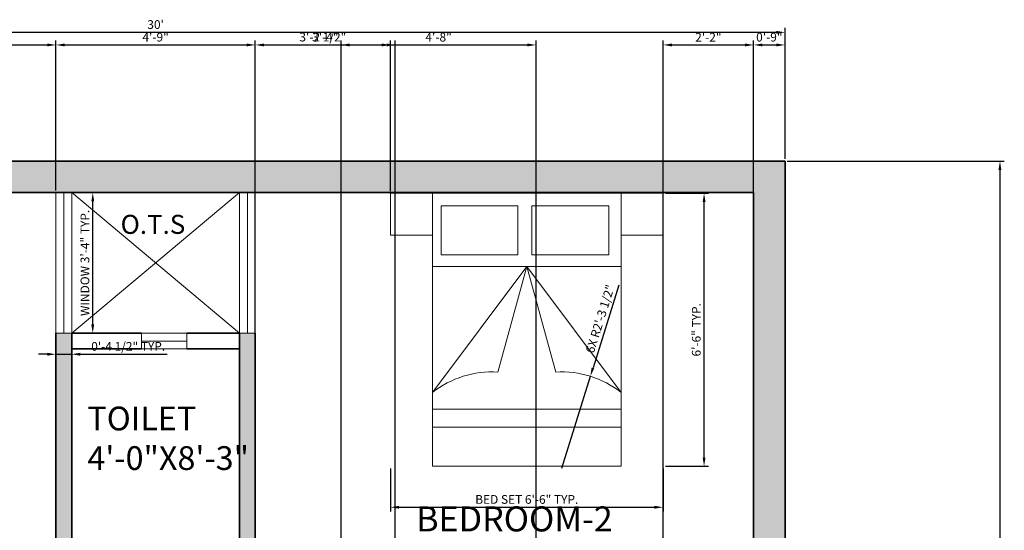
# Model space of a CAD drawing. Units: inches. Extents: x 2063 to 2524, y 2436 to 3097.
# Tile 4 of 4: x 2243 to 2524, y 2951 to 3097. Entities that reach past the tile are written whole.
import ezdxf

# ---------------------------------------------------------------- set-up
doc = ezdxf.new("R2010")
doc.units = ezdxf.units.IN
for name, color, linetype, lineweight in [('A-ANNO-DIMS', 2, 'Continuous', 18), ('A-AREA-IDEN', 7, 'Continuous', 18), ('A-FLOR-OPEN', 8, 'Continuous', 13), ('A-FURN', 8, 'Continuous', 18), ('A-GLAZ', 5, 'Continuous', 18), ('A-WALL', 7, 'Continuous', 35)]:
    doc.layers.add(name, color=color, linetype=linetype, lineweight=lineweight)
doc.layers.add('A-WALL-PATT', color=251, linetype='Continuous', lineweight=13, true_color=0x636466)
doc.styles.get("Standard").update_dxf_attribs({"font": 'arial.ttf'})
doc.dimstyles.new('ISO-25', dxfattribs={"dimtxt": 2.5, "dimasz": 2.5, "dimexe": 1.25, "dimexo": 0.625, "dimtad": 1, "dimlunit": 3, "dimtxsty": 'Standard', "dimcen": 2.5, "dimadec": 0, "dimazin": 0, "dimtfac": 1, "dimtmove": 0, "dimatfit": 3, "dimfxl": 1, "dimarcsym": 0})

# ---------------------------------------------------------------- blocks, each defined once
blk = doc.blocks.new('*D14')
at = {"layer": 'A-ANNO-DIMS', "color": 0, "lineweight": -2, "transparency": 16777216}
for p, q in [((2101.76, 3056.74), (2101.76, 3094.17)), ((2104.26, 3092.92), (2459.26, 3092.92)), ((2461.76, 3056.74), (2461.76, 3094.17))]:
    blk.add_line(p, q, dxfattribs=at)
at = {"layer": 'A-ANNO-DIMS', "color": 0, "transparency": 16777216}
for points in [[(2104.26, 3093.34), (2104.26, 3092.5), (2101.76, 3092.92)], [(2459.26, 3093.34), (2459.26, 3092.5), (2461.76, 3092.92)]]:
    blk.add_solid(points, dxfattribs=at)
at = {"layer": 'Defpoints', "color": 0, "transparency": 16777216}
for p in [(2461.76, 3092.92), (2101.76, 3056.12), (2461.76, 3056.12)]:
    blk.add_point(p, dxfattribs=at)
at = {"layer": 'A-ANNO-DIMS', "color": 0, "transparency": 16777216, "insert": (2281.76, 3094.82), "char_height": 2.5, "attachment_point": 5}
blk.add_mtext("30'", dxfattribs=at)
blk = doc.blocks.new('*D15')
at = {"layer": 'A-ANNO-DIMS', "color": 0, "lineweight": -2, "transparency": 16777216}
for p, q in [((2462.39, 3056.12), (2524.46, 3056.12)), ((2523.21, 3053.62), (2523.21, 2494.62)), ((2462.39, 2492.12), (2524.46, 2492.12))]:
    blk.add_line(p, q, dxfattribs=at)
at = {"layer": 'A-ANNO-DIMS', "color": 0, "transparency": 16777216}
for points in [[(2522.79, 3053.62), (2523.62, 3053.62), (2523.21, 3056.12)], [(2522.79, 2494.62), (2523.62, 2494.62), (2523.21, 2492.12)]]:
    blk.add_solid(points, dxfattribs=at)
at = {"layer": 'Defpoints', "color": 0, "transparency": 16777216}
for p in [(2461.76, 3056.12), (2461.76, 2492.12), (2523.21, 2492.12)]:
    blk.add_point(p, dxfattribs=at)
at = {"layer": 'A-ANNO-DIMS', "color": 0, "transparency": 16777216, "insert": (2521.33, 2774.12), "char_height": 2.5, "attachment_point": 5, "rotation": 90}
blk.add_mtext("47'", dxfattribs=at)
blk = doc.blocks.new('BED-DOUBLE-WITH-NIGHTSTANDS')
for p, q in [((12, 78), (0, 78)), ((0, 78), (0, 66)), ((66, 78), (78, 78)), ((78, 78), (78, 66)), ((36.48, 74.39), (36.48, 60.42)), ((40.48, 74.39), (40.48, 60.42)), ((0, 66), (12, 66)), ((77, 66), (66, 66)), ((78, 66), (77, 66)), ((12, 57.08), (66, 57.08)), ((39, 57.08), (12, 21.08)), ((39, 57.08), (30.7, 26.92)), ((39, 57.08), (66, 21.08)), ((39, 57.08), (47.3, 26.92))]:
    blk.add_line(p, q)
for points in [[(12, 0), (66, 0), (66, 78), (12, 78)], [(12, 16.31), (66, 16.31), (66, 11.16), (12, 11.16)]]:
    blk.add_lwpolyline(points, close=True)
for points in [[(36.48, 60.42), (14.53, 60.42), (14.53, 74.39), (36.48, 74.39)], [(40.48, 74.39), (62.43, 74.39), (62.43, 60.42), (40.48, 60.42)]]:
    blk.add_lwpolyline(points)
for centre, start, end in [((29, -0.5), 86.4578, 128.2353), ((49, -0.5), 51.7647, 93.5422)]:
    blk.add_arc(centre, 27.47, start, end)
blk = doc.blocks.new('WIN-OTS-40IN')
for p, q in [((0, 40.15), (0, 0)), ((2.25, 0), (2.25, 40.15)), ((4.5, 40.15), (4.5, 0))]:
    blk.add_line(p, q)
blk = doc.blocks.new('*D20')
at = {"layer": 'A-ANNO-DIMS', "color": 0, "lineweight": -2, "transparency": 16777216}
for p, q in [((2348.9, 2968.31), (2348.9, 2955.98)), ((2426.9, 2968.31), (2426.9, 2955.98)), ((2351.4, 2957.23), (2424.4, 2957.23))]:
    blk.add_line(p, q, dxfattribs=at)
at = {"layer": 'A-ANNO-DIMS', "color": 0, "transparency": 16777216}
for points in [[(2351.4, 2957.65), (2351.4, 2956.82), (2348.9, 2957.23)], [(2424.4, 2957.65), (2424.4, 2956.82), (2426.9, 2957.23)]]:
    blk.add_solid(points, dxfattribs=at)
at = {"layer": 'Defpoints', "color": 0, "transparency": 16777216}
for p in [(2348.9, 2968.93), (2426.9, 2968.93), (2426.9, 2957.23)]:
    blk.add_point(p, dxfattribs=at)
at = {"layer": 'A-ANNO-DIMS', "color": 0, "transparency": 16777216, "insert": (2387.9, 2959.15), "char_height": 2.5, "attachment_point": 5}
blk.add_mtext('BED SET 6\'-6" TYP.', dxfattribs=at)
blk = doc.blocks.new('*D21')
at = {"layer": 'A-ANNO-DIMS', "color": 0, "lineweight": -2, "transparency": 16777216}
for p, q in [((2427.53, 3046.93), (2439.85, 3046.93)), ((2438.6, 2971.43), (2438.6, 3044.43)), ((2427.53, 2968.93), (2439.85, 2968.93))]:
    blk.add_line(p, q, dxfattribs=at)
at = {"layer": 'A-ANNO-DIMS', "color": 0, "transparency": 16777216}
for points in [[(2438.19, 3044.43), (2439.02, 3044.43), (2438.6, 3046.93)], [(2438.19, 2971.43), (2439.02, 2971.43), (2438.6, 2968.93)]]:
    blk.add_solid(points, dxfattribs=at)
at = {"layer": 'Defpoints', "color": 0, "transparency": 16777216}
for p in [(2426.9, 3046.93), (2438.6, 3046.93), (2426.9, 2968.93)]:
    blk.add_point(p, dxfattribs=at)
at = {"layer": 'A-ANNO-DIMS', "color": 0, "transparency": 16777216, "insert": (2436.7, 3007.93), "char_height": 2.5, "attachment_point": 5, "rotation": 90}
blk.add_mtext('6\'-6" TYP.', dxfattribs=at)
blk = doc.blocks.new('*D24')
at = {"layer": 'A-ANNO-DIMS', "color": 0, "lineweight": -2, "transparency": 16777216}
for p, q in [((2258.39, 3047.12), (2265.04, 3047.12)), ((2263.79, 3009.47), (2263.79, 3044.62)), ((2258.39, 3006.97), (2265.04, 3006.97))]:
    blk.add_line(p, q, dxfattribs=at)
at = {"layer": 'A-ANNO-DIMS', "color": 0, "transparency": 16777216}
for points in [[(2263.37, 3044.62), (2264.2, 3044.62), (2263.79, 3047.12)], [(2263.37, 3009.47), (2264.2, 3009.47), (2263.79, 3006.97)]]:
    blk.add_solid(points, dxfattribs=at)
at = {"layer": 'Defpoints', "color": 0, "transparency": 16777216}
for p in [(2257.76, 3047.12), (2263.79, 3047.12), (2257.76, 3006.97)]:
    blk.add_point(p, dxfattribs=at)
at = {"layer": 'A-ANNO-DIMS', "color": 0, "transparency": 16777216, "insert": (2261.87, 3027.04), "char_height": 2.5, "attachment_point": 5, "rotation": 90}
blk.add_mtext('WINDOW 3\'-4" TYP.', dxfattribs=at)
blk = doc.blocks.new('*D25')
at = {"layer": 'A-ANNO-DIMS', "color": 0, "lineweight": -2, "transparency": 16777216}
for p, q in [((2253.26, 3006.35), (2253.26, 2999.7)), ((2257.76, 3006.35), (2257.76, 2999.7)), ((2250.76, 3000.95), (2248.26, 3000.95)), ((2253.26, 3000.95), (2257.76, 3000.95)), ((2260.26, 3000.95), (2285.08, 3000.95))]:
    blk.add_line(p, q, dxfattribs=at)
at = {"layer": 'A-ANNO-DIMS', "color": 0, "transparency": 16777216}
for points in [[(2250.76, 3001.37), (2250.76, 3000.53), (2253.26, 3000.95)], [(2260.26, 3001.37), (2260.26, 3000.53), (2257.76, 3000.95)]]:
    blk.add_solid(points, dxfattribs=at)
at = {"layer": 'Defpoints', "color": 0, "transparency": 16777216}
for p in [(2253.26, 3006.97), (2257.76, 3006.97), (2257.76, 3000.95)]:
    blk.add_point(p, dxfattribs=at)
at = {"layer": 'A-ANNO-DIMS', "color": 0, "transparency": 16777216, "insert": (2273.92, 3002.87), "char_height": 2.5, "attachment_point": 5}
blk.add_mtext('0\'-4 1/2" TYP.', dxfattribs=at)
blk = doc.blocks.new('*D32')
at = {"layer": 'A-ANNO-DIMS', "color": 0, "lineweight": -2, "transparency": 16777216}
for p, q in [((2101.76, 3056.74), (2101.76, 3090.57)), ((2104.26, 3089.32), (2250.76, 3089.32)), ((2253.26, 3047.74), (2253.26, 3090.57))]:
    blk.add_line(p, q, dxfattribs=at)
at = {"layer": 'A-ANNO-DIMS', "color": 0, "transparency": 16777216}
for points in [[(2104.26, 3089.73), (2104.26, 3088.9), (2101.76, 3089.32)], [(2250.76, 3089.73), (2250.76, 3088.9), (2253.26, 3089.32)]]:
    blk.add_solid(points, dxfattribs=at)
at = {"layer": 'Defpoints', "color": 0, "transparency": 16777216}
for p in [(2253.26, 3089.32), (2101.76, 3056.12), (2253.26, 3047.12)]:
    blk.add_point(p, dxfattribs=at)
at = {"layer": 'A-ANNO-DIMS', "color": 0, "transparency": 16777216, "insert": (2177.51, 3091.24), "char_height": 2.5, "attachment_point": 5}
blk.add_mtext('12\'-7 1/2"', dxfattribs=at)
blk = doc.blocks.new('*D33')
at = {"layer": 'A-ANNO-DIMS', "color": 0, "lineweight": -2, "transparency": 16777216}
for p, q in [((2253.26, 3047.74), (2253.26, 3090.57)), ((2255.76, 3089.32), (2307.76, 3089.32)), ((2310.26, 3047.74), (2310.26, 3090.57))]:
    blk.add_line(p, q, dxfattribs=at)
at = {"layer": 'A-ANNO-DIMS', "color": 0, "transparency": 16777216}
for points in [[(2255.76, 3089.73), (2255.76, 3088.9), (2253.26, 3089.32)], [(2307.76, 3089.73), (2307.76, 3088.9), (2310.26, 3089.32)]]:
    blk.add_solid(points, dxfattribs=at)
at = {"layer": 'Defpoints', "color": 0, "transparency": 16777216}
for p in [(2310.26, 3089.32), (2253.26, 3047.12), (2310.26, 3047.12)]:
    blk.add_point(p, dxfattribs=at)
at = {"layer": 'A-ANNO-DIMS', "color": 0, "transparency": 16777216, "insert": (2281.76, 3091.22), "char_height": 2.5, "attachment_point": 5}
blk.add_mtext('4\'-9"', dxfattribs=at)
blk = doc.blocks.new('*D37')
at = {"layer": 'A-ANNO-DIMS', "color": 0, "lineweight": -2, "transparency": 16777216}
for p, q in [((2452.76, 3047.74), (2452.76, 3090.57)), ((2455.26, 3089.32), (2459.26, 3089.32)), ((2461.76, 3056.74), (2461.76, 3090.57))]:
    blk.add_line(p, q, dxfattribs=at)
at = {"layer": 'A-ANNO-DIMS', "color": 0, "transparency": 16777216}
for points in [[(2455.26, 3089.73), (2455.26, 3088.9), (2452.76, 3089.32)], [(2459.26, 3089.73), (2459.26, 3088.9), (2461.76, 3089.32)]]:
    blk.add_solid(points, dxfattribs=at)
at = {"layer": 'Defpoints', "color": 0, "transparency": 16777216}
for p in [(2461.76, 3089.32), (2461.76, 3056.12), (2452.76, 3047.12)]:
    blk.add_point(p, dxfattribs=at)
at = {"layer": 'A-ANNO-DIMS', "color": 0, "transparency": 16777216, "insert": (2457.26, 3091.22), "char_height": 2.5, "attachment_point": 5}
blk.add_mtext('0\'-9"', dxfattribs=at)
blk = doc.blocks.new('*D38')
at = {"layer": 'A-ANNO-DIMS', "color": 0, "lineweight": -2, "transparency": 16777216}
for p, q in [((2310.26, 2812.24), (2310.26, 3090.57)), ((2312.76, 3089.32), (2347.8, 3089.32)), ((2350.3, 2812.24), (2350.3, 3090.57))]:
    blk.add_line(p, q, dxfattribs=at)
at = {"layer": 'A-ANNO-DIMS', "color": 0, "transparency": 16777216}
for points in [[(2312.76, 3089.73), (2312.76, 3088.9), (2310.26, 3089.32)], [(2347.8, 3089.73), (2347.8, 3088.9), (2350.3, 3089.32)]]:
    blk.add_solid(points, dxfattribs=at)
at = {"layer": 'Defpoints', "color": 0, "transparency": 16777216}
for p in [(2350.3, 3089.32), (2310.26, 2811.62), (2350.3, 2811.62)]:
    blk.add_point(p, dxfattribs=at)
at = {"layer": 'A-ANNO-DIMS', "color": 0, "transparency": 16777216, "insert": (2330.28, 3091.22), "char_height": 2.5, "attachment_point": 5}
blk.add_mtext('3\'-4"', dxfattribs=at)
blk = doc.blocks.new('*D39')
at = {"layer": 'A-ANNO-DIMS', "color": 0, "lineweight": -2, "transparency": 16777216}
for p, q in [((2426.9, 2762.84), (2426.9, 3090.57)), ((2429.4, 3089.32), (2450.26, 3089.32)), ((2452.76, 2762.84), (2452.76, 3090.57))]:
    blk.add_line(p, q, dxfattribs=at)
at = {"layer": 'A-ANNO-DIMS', "color": 0, "transparency": 16777216}
for points in [[(2429.4, 3089.73), (2429.4, 3088.9), (2426.9, 3089.32)], [(2450.26, 3089.73), (2450.26, 3088.9), (2452.76, 3089.32)]]:
    blk.add_solid(points, dxfattribs=at)
at = {"layer": 'Defpoints', "color": 0, "transparency": 16777216}
for p in [(2452.76, 3089.32), (2426.9, 2762.21), (2452.76, 2762.21)]:
    blk.add_point(p, dxfattribs=at)
at = {"layer": 'A-ANNO-DIMS', "color": 0, "transparency": 16777216, "insert": (2439.83, 3091.2), "char_height": 2.5, "attachment_point": 5}
blk.add_mtext('2\'-2"', dxfattribs=at)
blk = doc.blocks.new('*D47')
at = {"layer": 'A-ANNO-DIMS', "color": 0, "lineweight": -2, "transparency": 16777216}
for p, q in [((2310.26, 3047.74), (2310.26, 3090.57)), ((2312.76, 3089.32), (2346.4, 3089.32)), ((2348.9, 3047.56), (2348.9, 3090.57))]:
    blk.add_line(p, q, dxfattribs=at)
at = {"layer": 'A-ANNO-DIMS', "color": 0, "transparency": 16777216}
for points in [[(2312.76, 3089.73), (2312.76, 3088.9), (2310.26, 3089.32)], [(2346.4, 3089.73), (2346.4, 3088.9), (2348.9, 3089.32)]]:
    blk.add_solid(points, dxfattribs=at)
at = {"layer": 'Defpoints', "color": 0, "transparency": 16777216}
for p in [(2348.9, 3089.32), (2310.26, 3047.12), (2348.9, 3046.93)]:
    blk.add_point(p, dxfattribs=at)
at = {"layer": 'A-ANNO-DIMS', "color": 0, "transparency": 16777216, "insert": (2329.58, 3091.24), "char_height": 2.5, "attachment_point": 5}
blk.add_mtext('3\'-2 1/2"', dxfattribs=at)
blk = doc.blocks.new('*D49')
at = {"layer": 'A-ANNO-DIMS', "color": 0, "lineweight": -2, "transparency": 16777216}
for p, q in [((2334.8, 2697.62), (2334.8, 3090.57)), ((2337.3, 3089.32), (2388.07, 3089.32)), ((2390.57, 2697.62), (2390.57, 3090.57))]:
    blk.add_line(p, q, dxfattribs=at)
at = {"layer": 'A-ANNO-DIMS', "color": 0, "transparency": 16777216}
for points in [[(2337.3, 3089.73), (2337.3, 3088.9), (2334.8, 3089.32)], [(2388.07, 3089.73), (2388.07, 3088.9), (2390.57, 3089.32)]]:
    blk.add_solid(points, dxfattribs=at)
at = {"layer": 'Defpoints', "color": 0, "transparency": 16777216}
for p in [(2390.57, 3089.32), (2334.8, 2696.99), (2390.57, 2696.99)]:
    blk.add_point(p, dxfattribs=at)
at = {"layer": 'A-ANNO-DIMS', "color": 0, "transparency": 16777216, "insert": (2362.68, 3091.22), "char_height": 2.5, "attachment_point": 5}
blk.add_mtext('4\'-8"', dxfattribs=at)
blk = doc.blocks.new('*D52')
at = {"layer": 'A-ANNO-DIMS', "color": 0, "lineweight": -2, "transparency": 16777216}
for p, q in [((2414.21, 3020.65), (2406.84, 2997.04)), ((2397.9, 2968.43), (2406.09, 2994.66))]:
    blk.add_line(p, q, dxfattribs=at)
at = {"layer": 'A-ANNO-DIMS', "color": 0, "transparency": 16777216}
blk.add_solid([(2406.44, 2997.17), (2407.24, 2996.92), (2406.09, 2994.66)], dxfattribs=at)
at = {"layer": 'Defpoints', "color": 0, "transparency": 16777216}
for p in [(2406.09, 2994.66), (2397.9, 2968.43)]:
    blk.add_point(p, dxfattribs=at)
at = {"layer": 'A-ANNO-DIMS', "color": 0, "transparency": 16777216, "insert": (2409.18, 3010.96), "char_height": 2.5, "attachment_point": 5, "rotation": 72.6528}
blk.add_mtext('6X R2\'-3 1/2"', dxfattribs=at)

msp = doc.modelspace()

# ---------------------------------------------------------------- hatches: boundary and pattern name
at = {"layer": 'A-WALL-PATT'}
h = msp.add_hatch(color=256, dxfattribs=at)
h.dxf.hatch_style = 1
h.paths.add_polyline_path([(2110.763, 2670.618), (2110.763, 2676.643), (2110.763, 3047.118), (2452.763, 3047.118), (2452.763, 2501.118), (2200.478, 2501.118), (2200.478, 2492.118), (2461.763, 2492.118), (2461.763, 3056.118), (2101.763, 3056.118), (2101.763, 2492.118), (2149.478, 2492.118), (2149.478, 2496.618), (2149.478, 2501.118), (2110.763, 2501.118)])
h.paths.add_polyline_path([(2257.763, 2675.118), (2257.255, 2675.091), (2253.255, 2675.091), (2213.255, 2675.091), (2151.474, 2675.107), (2151.474, 2674.543), (2151.474, 2670.618), (2253.263, 2670.618), (2253.263, 2501.118), (2257.763, 2501.118)], flags=17)
h.paths.add_polyline_path([(2310.263, 3006.972), (2305.763, 3006.972), (2305.763, 2920.067), (2301.763, 2920.067), (2301.759, 2920.067), (2301.759, 2920.063), (2301.759, 2916.063), (2301.759, 2915.567), (2305.763, 2915.567), (2305.763, 2903.118), (2314.3, 2903.118), (2314.3, 2903.618), (2314.3, 2907.618), (2310.263, 2907.618)], flags=17)
h.paths.add_polyline_path([(2257.763, 3006.972), (2253.263, 3006.972), (2253.263, 2907.618), (2249.263, 2907.618), (2249.258, 2907.618), (2249.258, 2907.597), (2249.258, 2903.597), (2249.258, 2903.118), (2257.763, 2903.118), (2257.763, 2915.567), (2271.759, 2915.567), (2271.759, 2916.063), (2271.759, 2920.067), (2257.763, 2920.067)], flags=17)
h.paths.add_polyline_path([(2213.258, 2907.618), (2110.763, 2907.618), (2110.763, 2903.118), (2213.258, 2903.118), (2213.258, 2903.597)], flags=17)
h.paths.add_polyline_path([(2411.763, 2907.618), (2350.3, 2907.618), (2350.3, 2903.618), (2350.3, 2903.118), (2407.264, 2903.118), (2411.763, 2903.118)], flags=17)
h.paths.add_polyline_path([(2260.327, 2964.034), (2307.905, 2964.034), (2307.905, 2989.359), (2260.327, 2989.359)], flags=25)

# ---------------------------------------------------------------- linework, layer by layer
at = {"layer": 'A-FLOR-OPEN'}
for p, q in [((2257.763, 3047.118), (2305.763, 3006.972)), ((2305.763, 3047.118), (2257.763, 3006.972))]:
    msp.add_line(p, q, dxfattribs=at)
at = {"layer": 'A-GLAZ'}
for p, q in [((2257.763, 3006.972), (2253.263, 3006.972)), ((2277.709, 3004.722), (2277.709, 3006.972)), ((2277.709, 3006.972), (2277.709, 3002.472)), ((2290.709, 3006.972), (2277.709, 3006.972)), ((2289.709, 3004.722), (2277.709, 3004.722)), ((2290.709, 3004.722), (2289.709, 3004.722)), ((2290.709, 3006.972), (2290.709, 3002.472)), ((2290.709, 3002.472), (2290.709, 3004.722)), ((2305.763, 3006.972), (2310.263, 3006.972)), ((2290.709, 3002.472), (2277.709, 3002.472))]:
    msp.add_line(p, q, dxfattribs=at)
at = {"layer": 'A-WALL'}
for p, q in [((2101.763, 3056.118), (2461.763, 3056.118)), ((2461.763, 3056.118), (2461.763, 2492.118)), ((2110.763, 3047.118), (2452.763, 3047.118)), ((2452.763, 3047.118), (2452.763, 2501.118)), ((2253.263, 2907.618), (2253.263, 3006.972)), ((2277.709, 3006.972), (2257.763, 3006.972)), ((2257.763, 2920.067), (2257.763, 3006.972)), ((2305.763, 3006.972), (2290.709, 3006.972)), ((2305.763, 3006.972), (2305.763, 2920.067)), ((2310.263, 3006.972), (2310.263, 2907.618)), ((2277.709, 3002.472), (2257.763, 3002.472)), ((2305.763, 3002.472), (2290.709, 3002.472))]:
    msp.add_line(p, q, dxfattribs=at)

# ---------------------------------------------------------------- block references
at = {"layer": 'A-FURN'}
msp.add_blockref('BED-DOUBLE-WITH-NIGHTSTANDS', (2348.905, 2968.933), dxfattribs=at)
at = {"layer": 'A-GLAZ'}
msp.add_blockref('WIN-OTS-40IN', (2253.263, 3006.972), dxfattribs=at)
at = {"layer": 'A-GLAZ', "rotation": 180}
msp.add_blockref('WIN-OTS-40IN', (2310.264, 3047.118), dxfattribs=at)

# ---------------------------------------------------------------- texts
at = {"layer": 'A-AREA-IDEN', "attachment_point": 1}
for s, width, gutter_width, insert, char_height in [('O.T.S ', 7.82826, 27.18, (2271.749, 3040.778), 5.436), ('BEDROOM-2\\P11\'0"X12\'-3"', 18.93706, 35.717, (2356.274, 2957.479), 7.1434)]:
    msp.add_mtext_dynamic_manual_height_columns(s, width=width, gutter_width=gutter_width, heights=[0], dxfattribs=dict(at, insert=insert, char_height=char_height))
at = {"layer": 'A-AREA-IDEN', "insert": (2262.246, 2985.987), "char_height": 6.78682, "attachment_point": 1}
msp.add_mtext('TOILET\\P4\'-0"X8\'-3"', dxfattribs=at)

# ---------------------------------------------------------------- dimensions: what is measured, and where the dimension line sits
at = {"layer": 'A-ANNO-DIMS'}
for base, p1, p2, override, picture, middle in [((2461.763, 3092.92), (2101.763, 3056.118), (2461.763, 3056.118), {"dimclrd": 0, "dimclre": 0, "dimclrt": 0}, '*D14', (2281.763, 3094.823)), ((2253.263, 3089.318), (2101.763, 3056.118), (2253.263, 3047.118), {"dimdec": 1, "dimlfac": 1, "dimrnd": 0, "dimzin": 1, "dimdsep": 46, "dimlunit": 4, "dimfrac": 2}, '*D32', (2177.513, 3091.235)), ((2348.905, 3089.318), (2310.263, 3047.118), (2348.905, 3046.933), {"dimdec": 1, "dimlfac": 1, "dimrnd": 0, "dimzin": 1, "dimdsep": 46, "dimlunit": 4, "dimfrac": 2}, '*D47', (2329.584, 3091.236)), ((2310.263, 3089.318), (2253.263, 3047.118), (2310.263, 3047.118), {"dimdec": 1, "dimlfac": 1, "dimrnd": 0, "dimzin": 1, "dimdsep": 46, "dimlunit": 4, "dimfrac": 2}, '*D33', (2281.763, 3091.219)), ((2350.3, 3089.318), (2310.263, 2811.618), (2350.3, 2811.618), {"dimdec": 1, "dimlfac": 1, "dimrnd": 0, "dimzin": 1, "dimdsep": 46, "dimlunit": 4, "dimfrac": 2}, '*D38', (2330.282, 3091.22)), ((2390.571, 3089.318), (2334.798, 2696.991), (2390.571, 2696.991), {"dimdec": 1, "dimlfac": 1, "dimrnd": 0, "dimzin": 1, "dimdsep": 46, "dimlunit": 4, "dimfrac": 2}, '*D49', (2362.685, 3091.219)), ((2452.763, 3089.318), (2426.899, 2762.214), (2452.763, 2762.214), {"dimdec": 1, "dimlfac": 1, "dimrnd": 0, "dimzin": 1, "dimdsep": 46, "dimlunit": 4, "dimfrac": 2}, '*D39', (2439.831, 3091.198)), ((2461.763, 3089.318), (2452.763, 3047.118), (2461.763, 3056.118), {"dimdec": 1, "dimlfac": 1, "dimrnd": 0, "dimzin": 1, "dimdsep": 46, "dimlunit": 4, "dimfrac": 2}, '*D37', (2457.263, 3091.219))]:
    dim = msp.add_linear_dim(base=base, p1=p1, p2=p2, dimstyle='ISO-25', override=override, dxfattribs=at)
    dim.commit()
    dim.dimension.update_dxf_attribs({"geometry": picture, "text_midpoint": middle})
dim = msp.add_linear_dim(base=(2523.206, 2492.118), p1=(2461.763, 3056.118), p2=(2461.763, 2492.118), angle=90, dimstyle='ISO-25', override={"dimclrd": 0, "dimclre": 0, "dimclrt": 0}, dxfattribs=at)
dim.commit()
dim.dimension.update_dxf_attribs({"geometry": '*D15', "text_midpoint": (2521.331, 2774.118)})
for base, p1, p2, text, picture, middle in [((2263.785, 3047.118), (2257.763, 3006.972), (2257.763, 3047.118), 'WINDOW <> TYP.', '*D24', (2261.866, 3027.045)), ((2438.605, 3046.933), (2426.905, 2968.933), (2426.905, 3046.933), '<> TYP.', '*D21', (2436.703, 3007.933))]:
    dim = msp.add_linear_dim(base=base, p1=p1, p2=p2, angle=90, text=text, dimstyle='ISO-25', override={"dimdec": 1, "dimlfac": 1, "dimrnd": 0, "dimzin": 1, "dimdsep": 46, "dimlunit": 4, "dimfrac": 2}, dxfattribs=at)
    dim.commit()
    dim.dimension.update_dxf_attribs({"geometry": picture, "text_midpoint": middle})
dim = msp.add_radius_dim(center=(2397.903, 2968.434), mpoint=(2406.094, 2994.656), text='6X <>', dimstyle='ISO-25', override={"dimdec": 1, "dimlfac": 1, "dimrnd": 0, "dimzin": 1, "dimdsep": 46, "dimlunit": 4, "dimfrac": 2}, dxfattribs=at)
dim.commit()
dim.dimension.update_dxf_attribs({"geometry": '*D52', "text_midpoint": (2411.008, 3010.389), "dimtype": 164})
for base, p1, p2, text, picture, middle in [((2257.763, 3000.95), (2253.263, 3006.972), (2257.763, 3006.972), '<> TYP.', '*D25', (2273.921, 3002.868)), ((2426.905, 2957.233), (2348.905, 2968.933), (2426.905, 2968.933), 'BED SET <> TYP.', '*D20', (2387.905, 2959.151))]:
    dim = msp.add_linear_dim(base=base, p1=p1, p2=p2, text=text, dimstyle='ISO-25', override={"dimdec": 1, "dimlfac": 1, "dimrnd": 0, "dimzin": 1, "dimdsep": 46, "dimlunit": 4, "dimfrac": 2}, dxfattribs=at)
    dim.commit()
    dim.dimension.update_dxf_attribs({"geometry": picture, "text_midpoint": middle})

doc.saveas('drawing.dxf')
